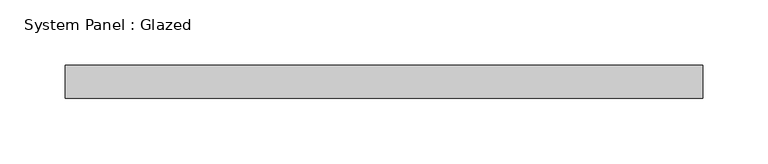
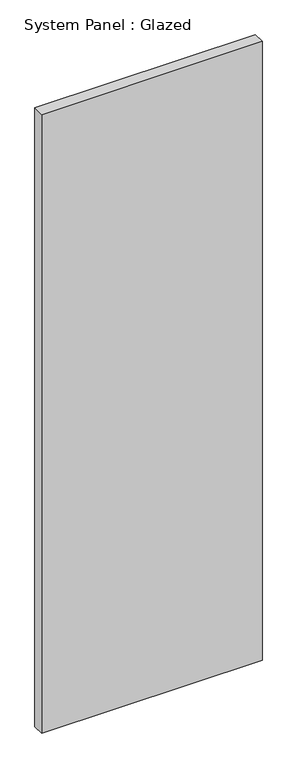
"""IFC4 building model written with IfcOpenShell, lengths in millimetres: plate geometry, System Panel : Glazed."""

from ifc_helpers import new_model, si_unit, origin, origin_with_axes, place, context, project, spatial, polyline, outline, extrude, source, transform, mapped, element, save


def system_panel_glazed_328f5a3b(model_context):
    return source(origin(), model_context, "Body", "SweptSolid", [
        extrude(outline(polyline([(244.475, 19.05), (-244.475, 19.05), (-244.475, 44.45), (244.475, 44.45), (244.475, 19.05)])), origin_with_axes(), (0.0, 0.0, 1.0), 1449.8375758),
    ])


if __name__ == "__main__":
    model = new_model("IFC4")
    model_context = context("Model", 3, world=origin())
    ifc_project = project(units=[si_unit("LENGTHUNIT", "METRE", prefix="MILLI")], contexts=[model_context])
    site = spatial("IfcSite", under=ifc_project)
    building = spatial("IfcBuilding", under=site)
    placement = place(None, origin())
    system_panel_glazed_shape = system_panel_glazed_328f5a3b(model_context)
    element("IfcPlate", 1, ObjectType="System Panel : Glazed", at=placement, inside=building, context=model_context, shape_type="MappedRepresentation", body=[
        mapped(system_panel_glazed_shape, transform((0.0, 0.0, 0.0), x_axis=(1.0, 0.0, 0.0), y_axis=(0.0, 1.0, 0.0), z_axis=(0.0, 0.0, 1.0))),
    ])
    save(model, "model.ifc")

# Revit data of these elements
# Type "System Panel : Glazed"
#   Construction Type Id = "GSP4R"
#   Analytic Construction = "1/8 in Pilkington single glazing"
#   Visual Light Transmittance = 0.9
#   Solar Heat Gain Coefficient = 0.86
#   Heat Transfer Coefficient (U) = 1.18115 BTU/(h·ft²·°F)
#   Define Thermal Properties by = 1
# Element 1 (IfcPlate, "System Panel : Glazed")
#   Materials on its faces: "Glass"
# Materials
#   "Glass": class "Glass", colour RGB 0 128 192, transparency 0.75, Description = "Soda Lime Glass", Cost = 0
